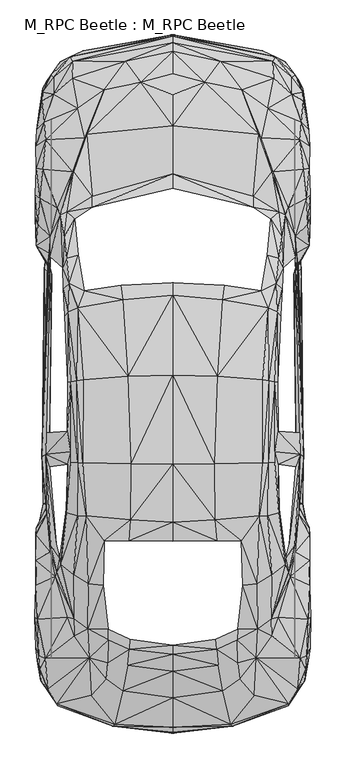
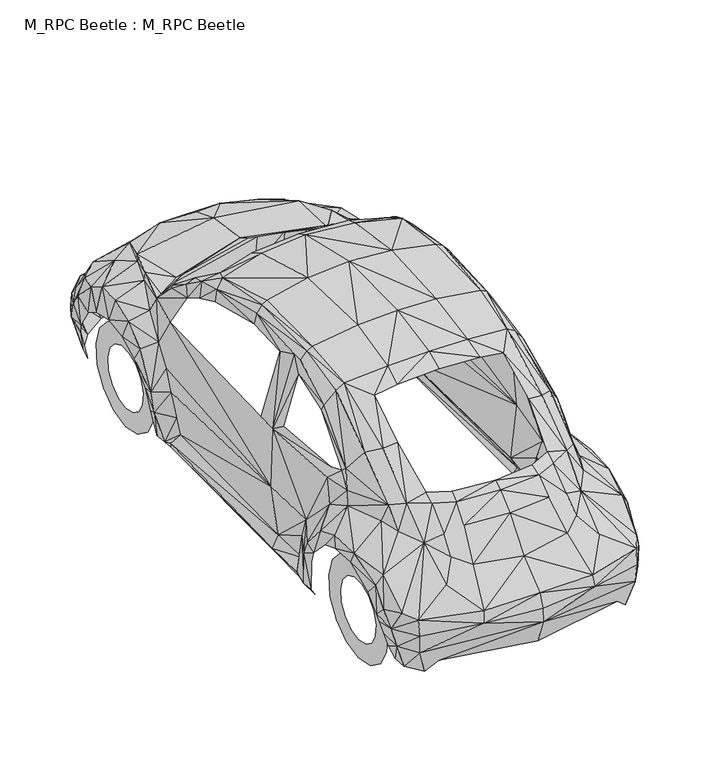
"""IFC4 building model written with IfcOpenShell, lengths in millimetres: proxy geometry, M_RPC Beetle : M_RPC Beetle."""

from ifc_helpers import new_model, si_unit, origin, place, context, project, spatial, triangles, source, transform, mapped, element, save


def m_rpc_beetle_m_rpc_beetle_b6d71803(model_context):
    return source(origin(), model_context, "Body", "Tessellation", [
        triangles([(0.0, -749.071574, 521.742899), (0.0, -720.6335569, 604.033443), (0.0, -697.1470545, 283.3282728), (0.0, -553.0728908, 738.9057701), (0.0, -753.760096, 438.7513078), (0.0, -253.8386484, 1040.4185434), (0.0, -401.3744104, 922.0218458), (0.0, -305.0182643, 1012.9445663), (0.0, 339.5469707, 1396.6602436), (0.0, 448.9171117, 1443.1075539), (0.0, 778.6050184, 1505.0664173), (0.0, 1285.8879353, 1510.4998066), (0.0, 1742.2541199, 1403.2768456), (0.0, 2432.6093651, 967.8556761), (0.0, 3132.1224815, 632.4714237), (0.0, 3003.4724854, 772.0323092), (0.0, 2706.0784286, 929.3833151), (0.0, 3166.3445206, 220.3177475), (0.0, 2885.1195351, 859.3180424), (0.0, 3224.7104347, 396.0724085), (0.0, 3181.1549538, 556.1401817), (0.0, 3216.1220055, 530.6379956), (-338.407687, -715.988855, 523.3642027), (-331.2653541, -702.6243364, 593.8676027), (-244.8997318, -218.1706584, 1034.7659815), (-249.1500901, -276.1420835, 1003.6112698), (-257.9137267, -368.4231514, 912.4695219), (-249.2377301, 343.0524253, 1381.9373051), (-285.431542, -511.8838351, 760.9462852), (-240.2988317, 460.3974792, 1427.552108), (-236.6180971, 781.4093531, 1494.4185207), (-652.9344915, -590.6250681, 370.7455024), (-540.4532759, -593.7361791, 283.6349946), (-181.3633847, 2956.2803078, 806.8677555), (-253.3566466, 1279.4466133, 1497.179108), (-380.1225826, -444.6667534, 798.8051662), (-371.1837024, -353.5687892, 889.7717068), (-368.2478714, -222.3771967, 1004.1371098), (-368.6422514, -160.8126769, 1037.3951088), (-390.4198829, 343.0962453, 1359.9406826), (-282.758631, 1714.4296555, 1400.2533382), (-397.6060358, 87.5486986, 1216.1732225), (-463.4209502, -538.1309249, 705.2972111), (-271.6726434, 3074.4140854, 663.1441154), (-476.0843851, -323.2904411, 850.4230185), (-464.0343939, 3087.9975586, 214.4022838), (-482.5694544, 95.8303334, 1204.2108713), (-485.3738254, -159.4104914, 1005.7583771), (-569.1103566, 3073.5815781, 547.1136251), (-493.874542, 483.577278, 1392.2346416), (-583.6579788, 3101.4935371, 522.400199), (-510.6130915, 3134.4011215, 369.6500387), (-392.1287902, 2913.6012268, 783.2935404), (-656.7905062, -598.249421, 480.4223834), (-660.6903408, -585.2354261, 576.6470695), (-562.669071, -200.2052034, 880.3069502), (-560.43436, -101.5266881, 987.8367239), (-512.8040188, 786.711355, 1449.4173431), (-542.1621832, 485.1109417, 1360.7731899), (-564.3779783, 148.6750366, 1173.0999796), (-608.8972449, -561.6174273, 218.6088402), (-511.6209151, 1259.3779255, 1457.1731197), (-542.7756269, 785.2215477, 1431.62715), (-459.1705556, 2305.6242382, 949.6711029), (-601.448172, -92.8068806, 893.8030014), (-504.0842022, 1766.485635, 1321.8626289), (-546.4125415, 1253.8568962, 1442.4940739), (-603.419963, 501.4989312, 1279.4466133), (-580.5469042, 789.4281223, 1379.6588104), (-607.6265376, 520.2092717, 1235.979063), (-601.6672357, 965.9276688, 1337.9439148), (-712.9654203, -503.4269022, 590.8879881), (-543.0385468, 1671.1811325, 1362.0876446), (-490.9387473, 2659.6751564, 894.1096687), (-600.0459683, 778.6050184, 1308.1913704), (-598.468521, 1244.567347, 1344.6919041), (-640.008173, 208.2677382, 1063.2039986), (-680.8904886, -470.5194632, 218.8279221), (-538.8320086, 1968.0492039, 1181.3815962), (-581.3794478, 1249.0807343, 1402.7071129), (-644.9596149, 243.4537263, 1028.9820322), (-502.6819985, 2637.5907486, 866.5918716), (-661.1722881, 162.3463042, 955.8933249), (-690.7057325, -396.8611321, 226.9780968), (-559.5141764, 2176.4921494, 1011.849139), (-670.6370447, 140.9630437, 873.2960409), (-662.9250154, 324.5173285, 1010.1402317), (-615.5138105, 1624.5585423, 1262.9710201), (-595.0507064, 1647.2125374, 1322.1692963), (-589.8363444, 1810.8295853, 1270.2885967), (-729.3095535, -482.3065707, 373.4622334), (-752.0950087, -454.7449536, 476.8731088), (-694.5179272, 315.5346282, 958.4347395), (-727.0748789, -327.5407994, 736.0575428), (-623.3572271, 1778.4479862, 1193.6068674), (-565.0352783, 2447.3761963, 934.772957), (-732.2892408, -394.1444012, 324.3420848), (-571.3888876, 2445.9300636, 884.7764448), (-699.1188818, 280.0419, 808.1822828), (-604.6907066, 1951.091518, 1171.2596123), (-587.8206971, 3015.1281693, 200.2490234), (-691.4068525, 574.6314222, 283.8102746), (-750.7366613, -381.2618663, 397.2555121), (-627.9581818, 1897.5456585, 1125.469602), (-602.8941593, 2217.067725, 949.8025629), (-619.8517725, 2074.2206303, 1075.9989298), (-710.949773, 550.0056361, 448.9171117), (-765.2404999, -360.5796985, 467.8465522), (-699.9952091, 763.1372126, 1016.187101), (-763.8382599, -313.4313409, 671.3819847), (-758.3609779, -391.2086065, 565.0352783), (-717.9606823, 496.6350929, 583.9647188), (-723.2188643, 461.5367629, 181.1004829), (-718.1359623, 554.8256181, 180.0050374), (-771.9884892, -342.0446016, 511.3579951), (-574.3247186, 2977.4883156, 683.0814159), (-731.2813808, 376.1351443, 185.3070212), (-541.5487395, 2807.2984131, 783.4688204), (-640.183453, 2199.9349045, 944.8949409), (-739.4315374, 551.9336434, 222.5524767), (-782.1104731, -268.9559124, 609.6421486), (-772.8209965, -106.1275973, 756.4330433), (-722.2110043, 958.3909195, 967.6803961), (-703.8074038, 810.6798775, 292.5300731), (-725.3221516, 835.6124399, 965.0075214), (-758.2734106, 370.7893224, 225.6197495), (-785.8788477, -90.0025187, 695.9639145), (-780.1824657, 80.9759712, 676.0266867), (-779.9195457, 89.5643369, 755.1622633), (-760.9024652, 444.4038334, 223.2973804), (-778.6050184, 192.2302905, 631.3321764), (-659.0690735, 2238.6701855, 850.3353785), (-771.4626492, 345.7253363, 426.4822165), (-774.7051838, 315.3593482, 502.0247349), (-781.7160931, 232.4115588, 696.3582945), (-719.7134096, 810.6360575, 185.964303), (-690.3552452, 1860.1249775, 294.1075386), (-697.1470545, 1960.2056419, 957.0763922), (-780.2701057, 377.6249516, 532.7412829), (-778.6488384, 417.2804163, 440.0220151), (-746.0043194, 820.1446341, 614.0678232), (-678.173794, 2886.7845497, 671.0752447), (-698.0233818, 2078.8215122, 757.3970106), (-640.051993, 3071.2590454, 391.9535102), (-713.4911877, 1919.5424263, 537.0792812), (-718.6617296, 1911.1731697, 193.1066541), (-705.6477711, 1983.2978371, 648.7279896), (-731.2813808, 1892.3751892, 233.5070043), (-674.4492393, 2909.8331429, 198.8030179), (-727.3815462, 2040.3052586, 190.0832013), (-722.1233643, 1974.7095531, 190.0832013), (-678.6557413, 2984.5867195, 540.8914395), (-700.0828491, 2817.5957497, 206.339749), (-696.8403145, 2993.6132034, 517.7554607), (-724.1390116, 2626.4609047, 788.1135223), (-699.5570091, 1883.7430126, 390.6389465), (-765.4157072, 2043.5477932, 362.8144094), (-742.2797647, 2459.3385475, 809.2338902), (-716.646155, 2967.1470863, 449.8372953), (-766.9494072, 2002.4902702, 376.836228), (-732.0701408, 2726.2786491, 728.1264862), (-771.6817492, 2086.0077015, 482.5694544), (-759.6317579, 2292.9609123, 780.6206657), (-769.5346418, 2144.7677776, 699.5131891), (-778.0791784, 2024.2239727, 495.1452856), (-742.9808121, 2848.7944267, 602.2807157), (-782.6363131, 2187.1400459, 616.8721579), (-740.0450174, 2920.3932541, 427.6653202), (-741.6224648, 2898.4841263, 520.1654517), (-750.9119413, 2806.3345184, 398.3509395), (-782.7677004, 2314.7385075, 681.1972286), (-778.6050184, 2464.4652695, 693.9921598), (-760.4204453, 2788.5004326, 455.5336773), (-774.7051838, 2684.6515388, 603.0694393), (-780.8835857, 2591.1871857, 666.7810301), (-743.1122721, 809.6720901, 220.5368294), (0.0, 2350.6693085, 1011.849139), (-459.1705556, 2241.4745201, 1007.2920044), (0.0, 1813.2396126, 1369.1424465), (-294.1513586, 1797.0267941, 1360.0720699), (-580.6345442, 850.2915585, 1382.7260651), (338.407687, -715.988855, 523.3642027), (331.2653541, -702.6243364, 593.8676027), (244.8997318, -218.1706584, 1034.7659815), (249.1500901, -276.1420835, 1003.6112698), (257.9137267, -368.4231514, 912.4695219), (249.2377301, 343.0524253, 1381.9373051), (285.431542, -511.8838351, 760.9462852), (240.2988317, 460.3974792, 1427.552108), (236.6180971, 781.4093531, 1494.4185207), (652.9344915, -590.6250681, 370.7455024), (540.4532759, -593.7361791, 283.6349946), (181.3633847, 2956.2803078, 806.8677555), (253.3566466, 1279.4466133, 1497.179108), (380.1225826, -444.6667534, 798.8051662), (371.1837024, -353.5687892, 889.7717068), (368.2478714, -222.3771967, 1004.1371098), (368.6422514, -160.8126769, 1037.3951088), (390.4198829, 343.0962453, 1359.9406826), (282.758631, 1714.4296555, 1400.2533382), (397.6060358, 87.5486986, 1216.1732225), (463.4209502, -538.1309249, 705.2972111), (271.6726434, 3074.4140854, 663.1441154), (476.0843851, -323.2904411, 850.4230185), (464.0343939, 3087.9975586, 214.4022838), (482.5694544, 95.8303334, 1204.2108713), (485.3738254, -159.4104914, 1005.7583771), (569.1103566, 3073.5815781, 547.1136251), (493.874542, 483.577278, 1392.2346416), (583.6579788, 3101.4935371, 522.400199), (510.6130915, 3134.4011215, 369.6500387), (392.1287902, 2913.6012268, 783.2935404), (656.7905062, -598.249421, 480.4223834), (660.6903408, -585.2354261, 576.6470695), (562.669071, -200.2052034, 880.3069502), (560.43436, -101.5266881, 987.8367239), (512.8040188, 786.711355, 1449.4173431), (542.1621832, 485.1109417, 1360.7731899), (564.3779783, 148.6750366, 1173.0999796), (608.8972449, -561.6174273, 218.6088402), (511.6209151, 1259.3779255, 1457.1731197), (542.7756269, 785.2215477, 1431.62715), (459.1705556, 2305.6242382, 949.6711029), (601.448172, -92.8068806, 893.8030014), (504.0842022, 1766.485635, 1321.8626289), (546.4125415, 1253.8568962, 1442.4940739), (603.419963, 501.4989312, 1279.4466133), (580.5469042, 789.4281223, 1379.6588104), (607.6265376, 520.2092717, 1235.979063), (601.6672357, 965.9276688, 1337.9439148), (712.9654203, -503.4269022, 590.8879881), (543.0385468, 1671.1811325, 1362.0876446), (490.9387473, 2659.6751564, 894.1096687), (600.0459683, 778.6050184, 1308.1913704), (598.468521, 1244.567347, 1344.6919041), (640.008173, 208.2677382, 1063.2039986), (680.9343086, -470.5194632, 218.8279221), (538.8320086, 1968.0492039, 1181.3815962), (581.3794478, 1249.0807343, 1402.7071129), (644.9596149, 243.4537263, 1028.9820322), (502.6819985, 2637.5907486, 866.5918716), (661.1722881, 162.3463042, 955.8933249), (690.7057325, -396.8611321, 226.9780968), (559.5141764, 2176.4921494, 1011.849139), (670.6370447, 140.9630437, 873.2960409), (662.9250154, 324.5173285, 1010.1402317), (615.5138105, 1624.5585423, 1262.9710201), (595.0507064, 1647.2125374, 1322.1692963), (589.8363444, 1810.8295853, 1270.2885967), (729.3095535, -482.3065707, 373.4622334), (752.0950087, -454.7449536, 476.8731088), (694.5179272, 315.5346282, 958.4347395), (727.0748789, -327.5407994, 736.0575428), (623.3572271, 1778.4479862, 1193.6068674), (565.0352783, 2447.3761963, 934.772957), (732.2892408, -394.1444012, 324.3420848), (571.3888876, 2445.9300636, 884.7764448), (699.1188818, 280.0419, 808.1822828), (604.6907066, 1951.091518, 1171.2596123), (587.8206971, 3015.1281693, 200.2490234), (691.4068525, 574.6314222, 283.8102746), (750.7366613, -381.2618663, 397.2555121), (627.9581818, 1897.5456585, 1125.469602), (602.8941593, 2217.067725, 949.8025629), (619.8517725, 2074.2206303, 1075.9989298), (710.949773, 550.0056361, 448.9171117), (765.2404999, -360.5796985, 467.8465522), (699.9952091, 763.1372126, 1016.187101), (763.8382599, -313.4313409, 671.3819847), (758.3609779, -391.2086065, 565.0352783), (717.9606823, 496.6350929, 583.9647188), (723.2188643, 461.5367629, 181.1004829), (718.1359623, 554.8256181, 180.0050374), (771.9884892, -342.0446016, 511.3579951), (574.3247186, 2977.4883156, 683.0814159), (731.2813808, 376.1351443, 185.3070212), (541.5487395, 2807.2984131, 783.4688204), (640.183453, 2199.9349045, 944.8949409), (739.4315374, 551.9336434, 222.5524767), (782.1104731, -268.9559124, 609.6421486), (772.8209965, -106.1275973, 756.4330433), (722.2548243, 958.3909195, 967.6803961), (703.8074038, 810.6798775, 292.5300731), (725.3221516, 835.6124399, 965.0075214), (758.2734106, 370.7893224, 225.6197495), (785.8788477, -90.0025187, 695.9639145), (780.1824657, 80.9759712, 676.0266867), (779.9633657, 89.5643369, 755.1622633), (760.9024652, 444.4038334, 223.2973804), (778.6050184, 192.2302905, 631.3321764), (659.0690735, 2238.6701855, 850.3353785), (771.4626492, 345.7253363, 426.4822165), (774.7051838, 315.3593482, 502.0247349), (781.7160931, 232.4115588, 696.3582945), (719.7134096, 810.6360575, 185.964303), (690.3552452, 1860.1249775, 294.1075386), (697.1470545, 1960.2056419, 957.0763922), (780.2701057, 377.6249516, 532.7412829), (778.6488384, 417.2804163, 440.0220151), (746.0043194, 820.1446341, 614.0678232), (678.173794, 2886.7845497, 671.0752447), (698.0233818, 2078.8215122, 757.3970106), (640.051993, 3071.2590454, 391.9535102), (713.4911877, 1919.5424263, 537.0792812), (718.6617296, 1911.1731697, 193.1066541), (705.6477711, 1983.2978371, 648.7279896), (731.2813808, 1892.3751892, 233.5070043), (674.4492393, 2909.8331429, 198.8030179), (727.3815462, 2040.3052586, 190.0832013), (722.1233643, 1974.7095531, 190.0832013), (678.6557413, 2984.5867195, 540.8914395), (700.0828491, 2817.5957497, 206.339749), (696.8403145, 2993.6132034, 517.7554607), (724.1390116, 2626.4609047, 788.1135223), (699.5570091, 1883.7430126, 390.6389465), (765.4157072, 2043.5477932, 362.8144094), (742.2797647, 2459.3385475, 809.2338902), (716.646155, 2967.1470863, 449.8372953), (766.9494072, 2002.4902702, 376.836228), (732.0701408, 2726.2786491, 728.1264862), (771.7255692, 2086.0077015, 482.5694544), (759.6317579, 2292.9609123, 780.6206657), (769.5346418, 2144.7677776, 699.5131891), (778.0791784, 2024.2239727, 495.1452856), (742.9808121, 2848.7944267, 602.2807157), (782.6363131, 2187.1400459, 616.8721579), (740.0450174, 2920.3932541, 427.6653202), (741.6224648, 2898.4841263, 520.1654517), (750.9119413, 2806.3345184, 398.3509395), (782.7677004, 2314.7385075, 681.1972286), (778.6050184, 2464.4652695, 693.9921598), (760.4204453, 2788.5004326, 455.5336773), (774.7051838, 2684.6515388, 603.0694393), (780.8835857, 2591.1871857, 666.7810301), (743.1122721, 809.6720901, 220.5368294), (459.1705556, 2241.4745201, 1007.2920044), (294.1513586, 1797.0267941, 1360.0720699), (580.6345442, 850.2915585, 1382.7260651), (-693.6415998, 2431.9082451, 0.0015117), (-693.6415998, 2431.9082451, 117.9161946), (-693.6415998, 2558.8496246, 26.9935036), (-693.6415998, 2509.4663017, 134.3918332), (-693.6415998, 2663.794091, 103.2371124), (-693.6415998, 2573.6600578, 181.0143508), (-693.6415998, 2728.6886765, 215.6307153), (-693.6415998, 2613.3154861, 249.7212399), (-693.6415998, 2742.2724403, 344.6752187), (-693.6415998, 2621.5972481, 328.5939328), (-693.6415998, 2702.1786667, 468.1109982), (-693.6415998, 2597.102813, 404.0050275), (-693.6415998, 2615.3310608, 564.5109644), (-693.6415998, 2544.0389008, 462.9404563), (-693.6415998, 2496.8028305, 617.3118113), (-693.6415998, 2471.5636734, 495.2344517), (-693.6415998, 2367.0135143, 617.3118113), (-693.6415998, 2392.2528168, 495.2344517), (-693.6415998, 2248.4854294, 564.5109644), (-693.6415998, 2319.7775894, 462.9404563), (-693.6415998, 2161.6378235, 468.1109982), (-693.6415998, 2266.7138226, 404.0050275), (-693.6415998, 2121.5441952, 344.6752187), (-693.6415998, 2242.2193874, 328.5939328), (-693.6415998, 2135.1278137, 215.6307153), (-693.6415998, 2250.501004, 249.7212399), (-693.6415998, 2200.0225445, 103.2371124), (-693.6415998, 2290.1564323, 181.0143508), (-693.6415998, 2304.9670109, 26.9935036), (-693.6415998, 2354.3500431, 134.3918332), (693.6415998, 2431.9082451, 0.0015117), (693.6415998, 2431.9082451, 117.9161946), (693.6415998, 2304.9670109, 26.9935036), (693.6415998, 2354.3500431, 134.3918332), (693.6415998, 2200.0225445, 103.2371124), (693.6415998, 2290.1564323, 181.0143508), (693.6415998, 2135.1278137, 215.6307153), (693.6415998, 2250.501004, 249.7212399), (693.6415998, 2121.5441952, 344.6752187), (693.6415998, 2242.2193874, 328.5939328), (693.6415998, 2161.6378235, 468.1109982), (693.6415998, 2266.7138226, 404.0050275), (693.6415998, 2248.4854294, 564.5109644), (693.6415998, 2319.7775894, 462.9404563), (693.6415998, 2367.0135143, 617.3118113), (693.6415998, 2392.2528168, 495.2344517), (693.6415998, 2496.8028305, 617.3118113), (693.6415998, 2471.5636734, 495.2344517), (693.6415998, 2615.3310608, 564.5109644), (693.6415998, 2544.0389008, 462.9404563), (693.6415998, 2702.1786667, 468.1109982), (693.6415998, 2597.102813, 404.0050275), (693.6415998, 2742.2724403, 344.6752187), (693.6415998, 2621.5972481, 328.5939328), (693.6415998, 2728.6886765, 215.6307153), (693.6415998, 2613.3154861, 249.7212399), (693.6415998, 2663.794091, 103.2371124), (693.6415998, 2573.6600578, 181.0143508), (693.6415998, 2558.8496246, 26.9935036), (693.6415998, 2509.4663017, 134.3918332), (-693.6415998, -13.5836322, 0.0015117), (-693.6415998, -13.5836322, 117.9161946), (-693.6415998, 113.3575975, 26.9935036), (-693.6415998, 63.9745244, 134.3918332), (-693.6415998, 218.3021002, 103.2371124), (-693.6415998, 128.1681397, 181.0143508), (-693.6415998, 283.1968128, 215.6307153), (-693.6415998, 167.8235862, 249.7212399), (-693.6415998, 296.7804495, 344.6752187), (-693.6415998, 176.1052209, 328.5939328), (-693.6415998, 256.6868212, 468.1109982), (-693.6415998, 151.6108585, 404.0050275), (-693.6415998, 169.8392153, 564.5109644), (-693.6415998, 98.5470553, 462.9404563), (-693.6415998, 51.3110713, 617.3118113), (-693.6415998, 26.0718098, 495.2344517), (-693.6415998, -78.4783402, 617.3118113), (-693.6415998, -53.2390741, 495.2344517), (-693.6415998, -197.0064706, 564.5109644), (-693.6415998, -125.7143196, 462.9404563), (-693.6415998, -283.8540765, 468.1109982), (-693.6415998, -178.7781137, 404.0050275), (-693.6415998, -323.9477048, 344.6752187), (-693.6415998, -203.2724762, 328.5939328), (-693.6415998, -310.3640862, 215.6307153), (-693.6415998, -194.9908414, 249.7212399), (-693.6415998, -245.4693737, 103.2371124), (-693.6415998, -155.335395, 181.0143508), (-693.6415998, -140.5248618, 26.9935036), (-693.6415998, -91.1417842, 134.3918332), (693.6415998, -13.5836322, 0.0015117), (693.6415998, -13.5836322, 117.9161946), (693.6415998, -140.5248618, 26.9935036), (693.6415998, -91.1417842, 134.3918332), (693.6415998, -245.4693737, 103.2371124), (693.6415998, -155.335395, 181.0143508), (693.6415998, -310.3640862, 215.6307153), (693.6415998, -194.9908414, 249.7212399), (693.6415998, -323.9477048, 344.6752187), (693.6415998, -203.2724762, 328.5939328), (693.6415998, -283.8540765, 468.1109982), (693.6415998, -178.7781137, 404.0050275), (693.6415998, -197.0064706, 564.5109644), (693.6415998, -125.7143196, 462.9404563), (693.6415998, -78.4783402, 617.3118113), (693.6415998, -53.2390741, 495.2344517), (693.6415998, 51.3110713, 617.3118113), (693.6415998, 26.0718098, 495.2344517), (693.6415998, 169.8392153, 564.5109644), (693.6415998, 98.5470553, 462.9404563), (693.6415998, 256.6868212, 468.1109982), (693.6415998, 151.6108585, 404.0050275), (693.6415998, 296.7804495, 344.6752187), (693.6415998, 176.1052209, 328.5939328), (693.6415998, 283.1968128, 215.6307153), (693.6415998, 167.8235862, 249.7212399), (693.6415998, 218.3021002, 103.2371124), (693.6415998, 128.1681397, 181.0143508), (693.6415998, 113.3575975, 26.9935036), (693.6415998, 63.9745244, 134.3918332)], [[67, 58, 62], [67, 63, 58], [53, 82, 74], [34, 17, 19], [118, 82, 53], [155, 98, 82], [155, 158, 98], [34, 74, 17], [172, 155, 175], [172, 158, 155], [159, 168, 169], [166, 142, 169], [175, 161, 174], [175, 155, 161], [142, 152, 169], [154, 169, 152], [160, 145, 165], [160, 156, 145], [162, 160, 165], [162, 157, 160], [34, 53, 74], [74, 96, 64], [82, 96, 74], [82, 98, 96], [36, 29, 27], [29, 43, 24], [23, 55, 54], [23, 24, 55], [23, 2, 24], [23, 1, 2], [5, 1, 23], [134, 140, 133], [134, 139, 140], [117, 130, 113], [117, 126, 130], [113, 120, 114], [113, 130, 120], [140, 112, 107], [140, 139, 112], [92, 108, 103], [91, 103, 97], [91, 92, 103], [61, 33, 32], [84, 78, 91], [84, 91, 97], [38, 26, 25], [77, 81, 83], [63, 50, 58], [63, 59, 50], [68, 63, 69], [68, 59, 63], [181, 75, 69], [74, 64, 17], [64, 14, 17], [64, 178, 14], [178, 177, 14], [34, 19, 16], [53, 34, 44], [21, 44, 15], [21, 49, 44], [44, 34, 15], [34, 16, 15], [22, 49, 21], [22, 51, 49], [20, 51, 22], [20, 52, 51], [18, 52, 20], [18, 46, 52], [51, 152, 49], [51, 154, 152], [101, 144, 46], [144, 52, 46], [101, 159, 144], [159, 169, 154], [101, 168, 159], [101, 149, 168], [149, 170, 168], [149, 153, 170], [168, 173, 169], [168, 170, 173], [49, 142, 116], [49, 152, 142], [49, 116, 44], [116, 142, 118], [161, 155, 118], [155, 82, 118], [142, 161, 118], [158, 132, 98], [158, 163, 132], [172, 163, 158], [172, 171, 163], [98, 119, 96], [98, 132, 119], [171, 164, 163], [171, 167, 164], [163, 143, 132], [163, 164, 143], [96, 105, 64], [96, 119, 105], [105, 178, 64], [105, 85, 178], [167, 165, 164], [167, 162, 165], [165, 143, 164], [165, 147, 143], [150, 160, 157], [150, 151, 160], [151, 156, 160], [151, 148, 137], [13, 35, 12], [13, 41, 35], [12, 31, 11], [12, 35, 31], [35, 58, 31], [35, 62, 58], [11, 30, 10], [11, 31, 30], [31, 50, 30], [31, 58, 50], [10, 28, 9], [10, 30, 28], [30, 40, 28], [30, 50, 40], [125, 75, 181], [125, 109, 75], [125, 87, 109], [125, 93, 87], [123, 141, 125], [137, 141, 156], [137, 124, 141], [148, 124, 137], [148, 176, 124], [146, 176, 148], [146, 136, 176], [141, 112, 125], [112, 93, 125], [112, 99, 93], [124, 112, 141], [124, 107, 112], [124, 102, 107], [176, 102, 124], [176, 120, 102], [136, 120, 176], [136, 114, 120], [47, 40, 50], [47, 42, 40], [48, 42, 47], [48, 39, 42], [57, 47, 60], [57, 48, 47], [60, 50, 59], [60, 47, 50], [59, 77, 60], [59, 68, 77], [77, 57, 60], [77, 83, 57], [70, 77, 68], [70, 81, 77], [75, 68, 69], [75, 70, 68], [26, 6, 25], [26, 8, 6], [27, 8, 26], [27, 7, 8], [29, 7, 27], [29, 4, 7], [24, 4, 29], [24, 2, 4], [32, 5, 23], [33, 5, 32], [33, 3, 5], [32, 23, 54], [55, 45, 72], [55, 24, 43], [99, 83, 93], [99, 86, 83], [135, 86, 99], [135, 129, 86], [131, 129, 135], [131, 128, 129], [93, 81, 87], [93, 83, 81], [128, 122, 129], [128, 127, 122], [122, 86, 129], [122, 65, 86], [86, 57, 83], [86, 65, 57], [127, 110, 122], [127, 121, 110], [110, 94, 122], [122, 94, 65], [94, 56, 65], [56, 57, 65], [56, 48, 57], [56, 45, 48], [94, 45, 56], [115, 110, 121], [115, 111, 110], [111, 94, 110], [111, 72, 94], [108, 92, 115], [92, 111, 115], [78, 32, 91], [78, 61, 32], [45, 38, 48], [45, 37, 38], [37, 26, 38], [37, 27, 26], [36, 27, 37], [134, 135, 139], [134, 131, 135], [139, 99, 112], [139, 135, 99], [126, 140, 130], [126, 133, 140], [130, 107, 120], [130, 140, 107], [120, 107, 102], [45, 36, 37], [92, 55, 72], [92, 54, 55], [91, 54, 92], [91, 32, 54], [92, 72, 111], [72, 45, 94], [43, 45, 55], [43, 36, 45], [43, 29, 36], [79, 90, 66], [79, 100, 90], [90, 73, 66], [85, 100, 79], [85, 106, 100], [85, 105, 106], [105, 119, 106], [95, 88, 89], [90, 89, 73], [89, 67, 73], [73, 67, 62], [89, 76, 80], [89, 80, 67], [88, 76, 89], [73, 35, 41], [73, 62, 35], [69, 63, 181], [80, 63, 67], [76, 71, 80], [146, 148, 151], [141, 147, 145], [151, 137, 156], [173, 166, 169], [173, 174, 166], [166, 174, 161], [166, 161, 142], [52, 144, 51], [144, 154, 51], [144, 159, 154], [116, 53, 44], [116, 118, 53], [119, 143, 138], [143, 119, 132], [143, 147, 138], [138, 104, 119], [119, 104, 106], [104, 100, 106], [104, 90, 100], [104, 95, 90], [95, 89, 90], [25, 39, 38], [38, 39, 48], [141, 138, 147], [156, 141, 145], [165, 145, 147], [41, 179, 180], [41, 13, 179], [66, 41, 180], [66, 73, 41], [123, 125, 71], [125, 181, 71], [71, 181, 80], [181, 63, 80], [138, 141, 123], [226, 221, 217], [226, 217, 222], [212, 233, 241], [193, 19, 17], [277, 212, 241], [314, 241, 257], [314, 257, 317], [193, 17, 233], [331, 334, 314], [331, 314, 317], [318, 328, 327], [325, 328, 301], [334, 333, 320], [334, 320, 314], [301, 328, 311], [313, 311, 328], [319, 324, 304], [319, 304, 315], [321, 324, 319], [321, 319, 316], [193, 233, 212], [233, 223, 255], [241, 233, 255], [241, 255, 257], [195, 186, 188], [188, 183, 202], [182, 213, 214], [182, 214, 183], [182, 183, 2], [182, 2, 1], [5, 182, 1], [293, 292, 299], [293, 299, 298], [276, 272, 289], [276, 289, 285], [272, 273, 279], [272, 279, 289], [299, 266, 271], [299, 271, 298], [251, 262, 267], [250, 256, 262], [250, 262, 251], [220, 191, 192], [243, 250, 237], [243, 256, 250], [197, 184, 185], [236, 242, 240], [222, 217, 209], [222, 209, 218], [227, 228, 222], [227, 222, 218], [338, 228, 234], [233, 17, 223], [223, 17, 14], [223, 14, 336], [336, 14, 177], [193, 16, 19], [212, 203, 193], [21, 15, 203], [21, 203, 208], [203, 15, 193], [193, 15, 16], [22, 21, 208], [22, 208, 210], [20, 22, 210], [20, 210, 211], [18, 20, 211], [18, 211, 205], [210, 208, 311], [210, 311, 313], [260, 205, 303], [303, 205, 211], [260, 303, 318], [318, 313, 328], [260, 318, 327], [260, 327, 308], [308, 327, 329], [308, 329, 312], [327, 328, 332], [327, 332, 329], [208, 275, 301], [208, 301, 311], [208, 203, 275], [275, 277, 301], [320, 277, 314], [314, 277, 241], [301, 277, 320], [317, 257, 291], [317, 291, 322], [331, 317, 322], [331, 322, 330], [257, 255, 278], [257, 278, 291], [330, 322, 323], [330, 323, 326], [322, 291, 302], [322, 302, 323], [255, 223, 264], [255, 264, 278], [264, 223, 336], [264, 336, 244], [326, 323, 324], [326, 324, 321], [324, 323, 302], [324, 302, 306], [309, 316, 319], [309, 319, 310], [310, 319, 315], [310, 296, 307], [13, 12, 194], [13, 194, 200], [12, 11, 190], [12, 190, 194], [194, 190, 217], [194, 217, 221], [11, 10, 189], [11, 189, 190], [190, 189, 209], [190, 209, 217], [10, 9, 187], [10, 187, 189], [189, 187, 199], [189, 199, 209], [284, 338, 234], [284, 234, 268], [284, 268, 246], [284, 246, 252], [282, 284, 300], [296, 315, 300], [296, 300, 283], [307, 296, 283], [307, 283, 335], [305, 307, 335], [305, 335, 295], [300, 284, 271], [271, 284, 252], [271, 252, 258], [283, 300, 271], [283, 271, 266], [283, 266, 261], [335, 283, 261], [335, 261, 279], [295, 335, 279], [295, 279, 273], [206, 209, 199], [206, 199, 201], [207, 206, 201], [207, 201, 198], [216, 219, 206], [216, 206, 207], [219, 218, 209], [219, 209, 206], [218, 219, 236], [218, 236, 227], [236, 219, 216], [236, 216, 242], [229, 227, 236], [229, 236, 240], [234, 228, 227], [234, 227, 229], [185, 184, 6], [185, 6, 8], [186, 185, 8], [186, 8, 7], [188, 186, 7], [188, 7, 4], [183, 188, 4], [183, 4, 2], [191, 182, 5], [192, 191, 5], [192, 5, 3], [191, 213, 182], [214, 231, 204], [214, 202, 183], [258, 252, 242], [258, 242, 245], [294, 258, 245], [294, 245, 288], [290, 294, 288], [290, 288, 287], [252, 246, 240], [252, 240, 242], [287, 288, 281], [287, 281, 286], [281, 288, 245], [281, 245, 224], [245, 242, 216], [245, 216, 224], [286, 281, 269], [286, 269, 280], [269, 281, 253], [281, 224, 253], [253, 224, 215], [215, 224, 216], [215, 216, 207], [215, 207, 204], [253, 215, 204], [274, 280, 269], [274, 269, 270], [270, 269, 253], [270, 253, 231], [267, 274, 251], [251, 274, 270], [237, 250, 191], [237, 191, 220], [204, 207, 197], [204, 197, 196], [196, 197, 185], [196, 185, 186], [195, 196, 186], [293, 298, 294], [293, 294, 290], [298, 271, 258], [298, 258, 294], [285, 289, 299], [285, 299, 292], [289, 279, 266], [289, 266, 299], [279, 261, 266], [204, 196, 195], [251, 231, 214], [251, 214, 213], [250, 251, 213], [250, 213, 191], [251, 270, 231], [231, 253, 204], [202, 214, 204], [202, 204, 195], [202, 195, 188], [238, 225, 249], [238, 249, 259], [249, 225, 232], [244, 238, 259], [244, 259, 265], [244, 265, 264], [264, 265, 278], [254, 248, 247], [249, 232, 248], [248, 232, 226], [232, 221, 226], [248, 239, 235], [248, 226, 239], [247, 248, 235], [232, 200, 194], [232, 194, 221], [228, 338, 222], [239, 226, 222], [235, 239, 230], [305, 310, 307], [300, 304, 306], [310, 315, 296], [332, 328, 325], [332, 325, 333], [325, 320, 333], [325, 301, 320], [211, 210, 303], [303, 210, 313], [303, 313, 318], [275, 203, 212], [275, 212, 277], [278, 297, 302], [302, 291, 278], [302, 297, 306], [297, 278, 263], [278, 265, 263], [263, 265, 259], [263, 259, 249], [263, 249, 254], [254, 249, 248], [184, 197, 198], [197, 207, 198], [300, 306, 297], [315, 304, 300], [324, 306, 304], [200, 337, 179], [200, 179, 13], [225, 337, 200], [225, 200, 232], [282, 230, 284], [284, 230, 338], [230, 239, 338], [338, 239, 222], [297, 282, 300], [339, 342, 341], [339, 340, 342], [341, 344, 343], [341, 342, 344], [343, 346, 345], [343, 344, 346], [345, 348, 347], [345, 346, 348], [347, 350, 349], [347, 348, 350], [349, 352, 351], [349, 350, 352], [351, 354, 353], [351, 352, 354], [353, 356, 355], [353, 354, 356], [355, 358, 357], [355, 356, 358], [357, 360, 359], [357, 358, 360], [359, 362, 361], [359, 360, 362], [361, 364, 363], [361, 362, 364], [363, 366, 365], [363, 364, 366], [365, 368, 367], [365, 366, 368], [367, 340, 339], [367, 368, 340], [369, 372, 371], [369, 370, 372], [371, 374, 373], [371, 372, 374], [373, 376, 375], [373, 374, 376], [375, 378, 377], [375, 376, 378], [377, 380, 379], [377, 378, 380], [379, 382, 381], [379, 380, 382], [381, 384, 383], [381, 382, 384], [383, 386, 385], [383, 384, 386], [385, 388, 387], [385, 386, 388], [387, 390, 389], [387, 388, 390], [389, 392, 391], [389, 390, 392], [391, 394, 393], [391, 392, 394], [393, 396, 395], [393, 394, 396], [395, 398, 397], [395, 396, 398], [397, 370, 369], [397, 398, 370], [399, 402, 401], [399, 400, 402], [401, 404, 403], [401, 402, 404], [403, 406, 405], [403, 404, 406], [405, 408, 407], [405, 406, 408], [407, 410, 409], [407, 408, 410], [409, 412, 411], [409, 410, 412], [411, 414, 413], [411, 412, 414], [413, 416, 415], [413, 414, 416], [415, 418, 417], [415, 416, 418], [417, 420, 419], [417, 418, 420], [419, 422, 421], [419, 420, 422], [421, 424, 423], [421, 422, 424], [423, 426, 425], [423, 424, 426], [425, 428, 427], [425, 426, 428], [427, 400, 399], [427, 428, 400], [429, 432, 431], [429, 430, 432], [431, 434, 433], [431, 432, 434], [433, 436, 435], [433, 434, 436], [435, 438, 437], [435, 436, 438], [437, 440, 439], [437, 438, 440], [439, 442, 441], [439, 440, 442], [441, 444, 443], [441, 442, 444], [443, 446, 445], [443, 444, 446], [445, 448, 447], [445, 446, 448], [447, 450, 449], [447, 448, 450], [449, 452, 451], [449, 450, 452], [451, 454, 453], [451, 452, 454], [453, 456, 455], [453, 454, 456], [455, 458, 457], [455, 456, 458], [457, 430, 429], [457, 458, 430]], closed=False),
    ])


if __name__ == "__main__":
    model = new_model("IFC4")
    model_context = context("Model", 3, world=origin())
    ifc_project = project(units=[si_unit("LENGTHUNIT", "METRE", prefix="MILLI")], contexts=[model_context])
    site = spatial("IfcSite", under=ifc_project)
    building = spatial("IfcBuilding", under=site)
    placement = place(None, origin())
    m_rpc_beetle_m_rpc_beetle_shape = m_rpc_beetle_m_rpc_beetle_b6d71803(model_context)
    element("IfcBuildingElementProxy", 1, Name="M_RPC Beetle : M_RPC Beetle", ObjectType="M_RPC Beetle : M_RPC Beetle", at=placement, inside=building, context=model_context, shape_type="MappedRepresentation", body=[
        mapped(m_rpc_beetle_m_rpc_beetle_shape, transform((0.0, 0.0, 0.0), x_axis=(1.0, 0.0, 0.0), y_axis=(0.0, 1.0, 0.0), z_axis=(0.0, 0.0, 1.0))),
    ])
    save(model, "model.ifc")

# Revit data of these elements
# Type "M_RPC Beetle : M_RPC Beetle"
#   built-in parameter 1005198 = "{2, 15},{39, RPC-16-0U6E-L4EG-ENH1-J3KF-SVEL-0TX4-C0},{1, 0},{1, 0},{2, 18},{1, 8},{5, Color},{1, 0},{1, 0},{3, 0.8},{3, 0.8},{3, 0.8},{1, 8},{7, BBoxMin},{1, 0},{1, 0},{1, 0},{1, 0},{1, 0},{1, 8},{7, BBoxMax},{1, 0},{1, 0},{1, 0},{1, 0},{1, 0},{2, 11},{9, RPCTypeId},{1, 0},{1, 0},{39, RPC-16-0U6E-L4EG-ENH1-J3KF-SVEL-0TX4-C0},{1, 6},{14, RPCPlantHeight},{1, 0},{1, 0},{4, 4.92},{2, 11},{7, keyword},{1, 0},{1, 0},{39, :RPCs:Auto_Economy/Midsize:Geometry:RPC},{2, 11},{8, category},{1, 0},{1, 0},{20, Auto_Economy/Midsize},{2, 11},{12, LocalizedUID},{1, 0},{1, 0},{13, VW Beetle [4]},{2, 14},{6, Height},{1, 0},{1, 0},{4, 4.92},{1, 2},{16, Cast Reflections},{1, 0},{1, 0},{1, 0},{1, 4},{12, Transparency},{1, 0},{1, 0},{2, 18},{1, 4},{7, Tinting},{1, 0},{1, 0},{2, 50},{1, 2},{11, Use Tinting},{1, 0},{1, 0},{1, 0},{1, 2},{13, License Plate},{1, 0},{1, 0},{1, 0},{2, 11},{21, License Plate Texture},{1, 0},{1, 0},{64, __RPC:/object data/textures/car/plate/textures/default/rgb/0/0/0},{2, 11},{23, i_License Plate Texture},{1, 0},{1, 0},{0, },{1, 2},{12, Custom Plate},{1, 0},{1, 0},{1, 0},{2, 11},{23, License Plate File Name},{1, 0},{1, 0},{0, },{21, assetlibrary_base.fbx},{1, 5},"
#   built-in parameter 1005195 = "RPC-16-0U6E-L4EG-ENH1-J3KF-SVEL-0TX4-C0"
#   Height = 0
